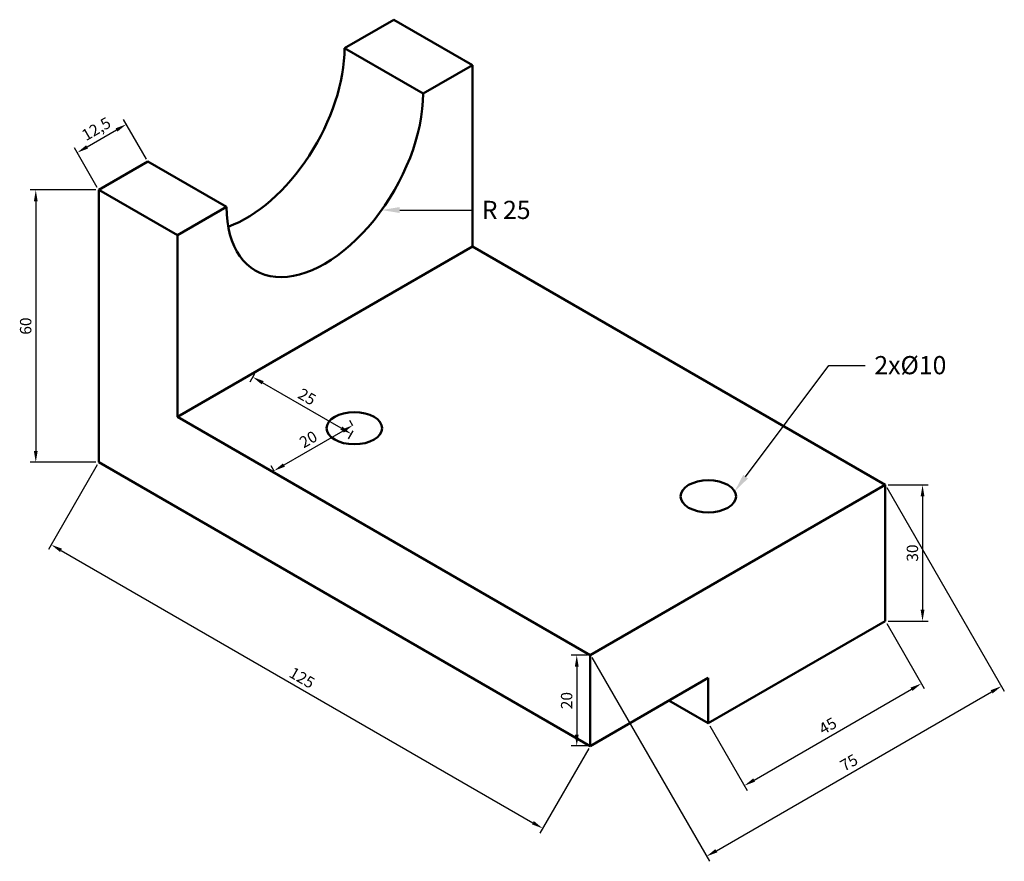
# Model space of a CAD drawing. Units: millimetres. Extents: x 163 to 380, y 64 to 249.
import ezdxf
from ezdxf import colors
from ezdxf.entities.mleader import LeaderData, LeaderLine
from ezdxf.math import Vec2, Vec3

# ---------------------------------------------------------------- set-up
doc = ezdxf.new("R2010")
doc.units = ezdxf.units.MM
for name, color, linetype, lineweight in [('M-DIMS', 2, 'Continuous', 25), ('M-OUTL', 7, 'Continuous', 50), ('M-TEXT', 3, 'Continuous', 25)]:
    doc.layers.add(name, color=color, linetype=linetype, lineweight=lineweight)
doc.styles.get("Standard").update_dxf_attribs({"font": 'arial.ttf'})
doc.dimstyles.new('ISO-25', dxfattribs={"dimtxt": 2.5, "dimasz": 2.5, "dimexe": 1.25, "dimexo": 0.625, "dimtad": 1, "dimtxsty": 'Standard', "dimcen": 2.5, "dimadec": 0, "dimazin": 0, "dimtfac": 1, "dimtmove": 0, "dimatfit": 3, "dimfxl": 1, "dimarcsym": 0})

# ---------------------------------------------------------------- blocks, each defined once
blk = doc.blocks.new('*D1')
at = {"layer": 'Defpoints', "color": 0, "transparency": 16777216}
for p in [(180.55, 211.41), (166.68, 151.41), (180.55, 151.41)]:
    blk.add_point(p, dxfattribs=at)
at = {"layer": 'M-DIMS', "color": 0, "lineweight": -2, "transparency": 16777216}
for p, q in [((179.92, 211.41), (165.43, 211.41)), ((166.68, 208.91), (166.68, 153.91)), ((179.92, 151.41), (165.43, 151.41))]:
    blk.add_line(p, q, dxfattribs=at)
at = {"layer": 'M-DIMS', "color": 0, "transparency": 16777216}
for points in [[(166.27, 208.91), (167.1, 208.91), (166.68, 211.41)], [(166.27, 153.91), (167.1, 153.91), (166.68, 151.41)]]:
    blk.add_solid(points, dxfattribs=at)
at = {"layer": 'M-DIMS', "color": 0, "transparency": 16777216, "insert": (164.78, 181.41), "char_height": 2.5, "attachment_point": 5, "rotation": 90}
blk.add_mtext('60', dxfattribs=at)
blk = doc.blocks.new('*D2')
at = {"layer": 'Defpoints', "color": 0, "transparency": 16777216}
for p in [(180.55, 151.41), (288.8, 88.91), (278.32, 70.76)]:
    blk.add_point(p, dxfattribs=at)
at = {"layer": 'M-DIMS', "color": 0, "lineweight": -2, "transparency": 16777216}
for p, q in [((180.23, 150.87), (169.45, 132.18)), ((172.24, 132.01), (276.16, 72.01)), ((288.49, 88.37), (277.7, 69.68))]:
    blk.add_line(p, q, dxfattribs=at)
at = {"layer": 'M-DIMS', "color": 0, "transparency": 16777216}
for points in [[(172.45, 132.37), (172.03, 131.65), (170.07, 133.26)], [(276.37, 72.37), (275.95, 71.65), (278.32, 70.76)]]:
    blk.add_solid(points, dxfattribs=at)
at = {"layer": 'M-DIMS', "color": 0, "transparency": 16777216, "insert": (225.15, 103.66), "char_height": 2.5, "attachment_point": 5, "rotation": 330}
blk.add_mtext('125', dxfattribs=at)
blk = doc.blocks.new('*D3')
at = {"layer": 'Defpoints', "color": 0, "transparency": 16777216}
for p in [(353.75, 116.41), (361.69, 102.66), (314.78, 93.91)]:
    blk.add_point(p, dxfattribs=at)
at = {"layer": 'M-DIMS', "color": 0, "lineweight": -2, "transparency": 16777216}
for p, q in [((354.06, 115.87), (362.31, 101.58)), ((324.88, 81.41), (359.52, 101.41)), ((315.09, 93.37), (323.34, 79.08))]:
    blk.add_line(p, q, dxfattribs=at)
at = {"layer": 'M-DIMS', "color": 0, "transparency": 16777216}
for points in [[(359.31, 101.78), (359.73, 101.05), (361.69, 102.66)], [(324.67, 81.78), (325.09, 81.05), (322.72, 80.16)]]:
    blk.add_solid(points, dxfattribs=at)
at = {"layer": 'M-DIMS', "color": 0, "transparency": 16777216, "insert": (341.25, 93.06), "char_height": 2.5, "attachment_point": 5, "rotation": 30}
blk.add_mtext('45', dxfattribs=at)
blk = doc.blocks.new('*D4')
at = {"layer": 'Defpoints', "color": 0, "transparency": 16777216}
for p in [(288.8, 108.91), (285.81, 88.91), (288.8, 88.91)]:
    blk.add_point(p, dxfattribs=at)
at = {"layer": 'M-DIMS', "color": 0, "lineweight": -2, "transparency": 16777216}
for p, q in [((288.18, 108.91), (284.56, 108.91)), ((285.81, 106.41), (285.81, 91.41)), ((288.18, 88.91), (284.56, 88.91))]:
    blk.add_line(p, q, dxfattribs=at)
at = {"layer": 'M-DIMS', "color": 0, "transparency": 16777216}
for points in [[(285.4, 106.41), (286.23, 106.41), (285.81, 108.91)], [(285.4, 91.41), (286.23, 91.41), (285.81, 88.91)]]:
    blk.add_solid(points, dxfattribs=at)
at = {"layer": 'M-DIMS', "color": 0, "transparency": 16777216, "insert": (283.91, 98.91), "char_height": 2.5, "attachment_point": 5, "rotation": 90}
blk.add_mtext('20', dxfattribs=at)
blk = doc.blocks.new('*D5')
at = {"layer": 'Defpoints', "color": 0, "transparency": 16777216}
for p in [(236.84, 158.91), (219.15, 149.54), (219.52, 148.91)]:
    blk.add_point(p, dxfattribs=at)
at = {"layer": 'M-DIMS', "color": 0, "lineweight": -2, "transparency": 16777216}
for p, q in [((236.53, 159.45), (235.85, 160.62)), ((234.31, 158.29), (221.32, 150.79)), ((219.21, 149.45), (218.53, 150.62))]:
    blk.add_line(p, q, dxfattribs=at)
at = {"layer": 'M-DIMS', "color": 0, "transparency": 16777216}
for points in [[(234.1, 158.65), (234.52, 157.93), (236.47, 159.54)], [(221.11, 151.15), (221.53, 150.43), (219.15, 149.54)]]:
    blk.add_solid(points, dxfattribs=at)
at = {"layer": 'M-DIMS', "color": 0, "transparency": 16777216, "insert": (226.86, 156.19), "char_height": 2.5, "attachment_point": 5, "rotation": 30}
blk.add_mtext('20', dxfattribs=at)
blk = doc.blocks.new('*D6')
at = {"layer": 'Defpoints', "color": 0, "transparency": 16777216}
for p in [(215.19, 171.41), (214.48, 170.18), (236.84, 158.91)]:
    blk.add_point(p, dxfattribs=at)
at = {"layer": 'M-DIMS', "color": 0, "lineweight": -2, "transparency": 16777216}
for p, q in [((214.88, 170.87), (213.85, 169.09)), ((233.96, 158.93), (216.64, 168.93)), ((236.53, 158.37), (235.5, 156.59))]:
    blk.add_line(p, q, dxfattribs=at)
at = {"layer": 'M-DIMS', "color": 0, "transparency": 16777216}
for points in [[(216.85, 169.29), (216.43, 168.56), (214.48, 170.18)], [(234.17, 159.29), (233.75, 158.56), (236.13, 157.68)]]:
    blk.add_solid(points, dxfattribs=at)
at = {"layer": 'M-DIMS', "color": 0, "transparency": 16777216, "insert": (226.25, 165.57), "char_height": 2.5, "attachment_point": 5, "rotation": 330}
blk.add_mtext('25', dxfattribs=at)
blk = doc.blocks.new('*D7')
at = {"layer": 'Defpoints', "color": 0, "transparency": 16777216}
for p in [(353.75, 146.41), (288.8, 108.91), (379.34, 102.09)]:
    blk.add_point(p, dxfattribs=at)
at = {"layer": 'M-DIMS', "color": 0, "lineweight": -2, "transparency": 16777216}
for p, q in [((354.06, 145.87), (379.96, 101.01)), ((289.11, 108.37), (315.01, 63.51)), ((316.55, 65.84), (377.17, 100.84))]:
    blk.add_line(p, q, dxfattribs=at)
at = {"layer": 'M-DIMS', "color": 0, "transparency": 16777216}
for points in [[(376.97, 101.2), (377.38, 100.48), (379.34, 102.09)], [(316.34, 66.2), (316.76, 65.48), (314.39, 64.59)]]:
    blk.add_solid(points, dxfattribs=at)
at = {"layer": 'M-DIMS', "color": 0, "transparency": 16777216, "insert": (345.91, 84.98), "char_height": 2.5, "attachment_point": 5, "rotation": 30}
blk.add_mtext('75', dxfattribs=at)
blk = doc.blocks.new('*D8')
at = {"layer": 'Defpoints', "color": 0, "transparency": 16777216}
for p in [(353.75, 146.41), (353.75, 116.41), (361.96, 116.41)]:
    blk.add_point(p, dxfattribs=at)
at = {"layer": 'M-DIMS', "color": 0, "lineweight": -2, "transparency": 16777216}
for p, q in [((354.38, 146.41), (363.21, 146.41)), ((361.96, 143.91), (361.96, 118.91)), ((354.38, 116.41), (363.21, 116.41))]:
    blk.add_line(p, q, dxfattribs=at)
at = {"layer": 'M-DIMS', "color": 0, "transparency": 16777216}
for points in [[(361.54, 143.91), (362.37, 143.91), (361.96, 146.41)], [(361.54, 118.91), (362.37, 118.91), (361.96, 116.41)]]:
    blk.add_solid(points, dxfattribs=at)
at = {"layer": 'M-DIMS', "color": 0, "transparency": 16777216, "insert": (360.05, 131.41), "char_height": 2.5, "attachment_point": 5, "rotation": 90}
blk.add_mtext('30', dxfattribs=at)
blk = doc.blocks.new('*D9')
at = {"layer": 'Defpoints', "color": 0, "transparency": 16777216}
for p in [(186.63, 225.87), (191.37, 217.66), (180.55, 211.41)]:
    blk.add_point(p, dxfattribs=at)
at = {"layer": 'M-DIMS', "color": 0, "lineweight": -2, "transparency": 16777216}
for p, q in [((191.06, 218.2), (186.01, 226.95)), ((177.97, 220.87), (184.47, 224.62)), ((180.23, 211.95), (175.18, 220.7))]:
    blk.add_line(p, q, dxfattribs=at)
at = {"layer": 'M-DIMS', "color": 0, "transparency": 16777216}
for points in [[(184.26, 224.98), (184.68, 224.26), (186.63, 225.87)], [(177.76, 221.23), (178.18, 220.51), (175.81, 219.62)]]:
    blk.add_solid(points, dxfattribs=at)
at = {"layer": 'M-DIMS', "color": 0, "transparency": 16777216, "insert": (180.16, 224.58), "char_height": 2.5, "attachment_point": 5, "rotation": 30}
blk.add_mtext('12,5', dxfattribs=at)

msp = doc.modelspace()

# ---------------------------------------------------------------- linework, layer by layer
at = {"layer": 'M-OUTL'}
for p, q in [((245.499, 248.907), (234.674, 242.657)), ((262.819, 238.907), (245.499, 248.907)), ((234.674, 242.657), (251.994, 232.657)), ((251.994, 232.657), (262.819, 238.907)), ((262.819, 198.907), (262.819, 238.907)), ((191.372, 217.657), (180.547, 211.407)), ((191.372, 217.657), (208.693, 207.657)), ((180.547, 151.407), (180.547, 211.407)), ((180.547, 211.407), (197.867, 201.407)), ((197.867, 201.407), (208.693, 207.657)), ((197.867, 201.407), (197.867, 161.407)), ((197.867, 161.407), (262.819, 198.907)), ((353.752, 146.407), (262.819, 198.907)), ((197.867, 161.407), (288.8, 108.907)), ((180.547, 151.407), (288.8, 88.907)), ((288.8, 108.907), (353.752, 146.407)), ((353.752, 116.407), (353.752, 146.407)), ((314.781, 93.907), (353.752, 116.407)), ((288.8, 108.907), (288.8, 88.907)), ((288.8, 88.907), (314.781, 103.907)), ((314.781, 103.907), (314.781, 93.907)), ((314.781, 93.907), (306.121, 98.907))]:
    msp.add_line(p, q, dxfattribs=at)
for centre, start_param in [((213.023, 230.157), 6.8844495), ((230.343, 220.157), 5.4977871)]:
    msp.add_ellipse(centre, major_axis=(-15.309, -26.517), ratio=0.5773503, start_param=start_param, end_param=8.6393798, dxfattribs=at)
for centre in [(236.839, 158.907), (314.781, 143.907)]:
    msp.add_ellipse(centre, major_axis=(-6.124, 0), ratio=0.5773503, dxfattribs=at)

# ---------------------------------------------------------------- dimensions: what is measured, and where the dimension line sits
at = {"layer": 'M-DIMS'}
for p1, p2, distance, picture, middle in [((180.547, 211.407), (191.372, 217.657), 9.479, '*D9', (180.156, 224.584)), ((236.839, 158.907), (215.188, 171.407), 1.423, '*D6', (226.253, 165.572)), ((236.839, 158.907), (219.518, 148.907), -0.729, '*D5', (226.863, 156.185)), ((180.547, 151.407), (288.8, 88.907), -20.951, '*D2', (225.149, 103.66)), ((288.8, 108.907), (353.752, 146.407), -51.174, '*D7', (345.915, 84.982)), ((314.781, 93.907), (353.752, 116.407), -15.869, '*D3', (341.253, 93.057))]:
    dim = msp.add_aligned_dim(p1=p1, p2=p2, distance=distance, dimstyle='ISO-25', override={"dimclrd": 0, "dimclre": 0, "dimclrt": 0}, dxfattribs=at)
    dim.commit()
    dim.dimension.update_dxf_attribs({"geometry": picture, "text_midpoint": middle})
for base, p1, p2, picture, middle in [((166.683, 151.407), (180.547, 211.407), (180.547, 151.407), '*D1', (164.782, 181.407)), ((361.956, 116.407), (353.752, 146.407), (353.752, 116.407), '*D8', (360.054, 131.407)), ((285.814, 88.907), (288.8, 108.907), (288.8, 88.907), '*D4', (283.912, 98.907))]:
    dim = msp.add_linear_dim(base=base, p1=p1, p2=p2, angle=90, dimstyle='ISO-25', override={"dimclrd": 0, "dimclre": 0, "dimclrt": 0}, dxfattribs=at)
    dim.commit()
    dim.dimension.update_dxf_attribs({"geometry": picture, "text_midpoint": middle})

# ---------------------------------------------------------------- leaders
at = {"layer": 'M-TEXT'}
ml = msp.add_multileader_mtext('Standard', dxfattribs=at)
ml.set_content('R 25', color=256)
ml.set_leader_properties()
ml.build(insert=Vec2(0, 0))
ctx = ml.context
ctx.base_point, ctx.plane_origin = Vec3(262.892, 206.973), Vec3(242.852, 206.973)
notes = []
notes.append((ctx, [(0, (1, 1, 0), (254.892, 206.973), (1, 0), 8, [(0, [(242.852, 206.973)], 0, [])])]))
ctx.mtext.insert, ctx.mtext.flow_direction = Vec3(264.892, 209.007), 5
ml = msp.add_multileader_mtext('Standard', dxfattribs=at)
ml.set_content('2x%%C10', color=256)
ml.set_leader_properties()
ml.build(insert=Vec2(0, 0))
ctx = ml.context
ctx.base_point, ctx.plane_origin = Vec3(349.353, 172.726), Vec3(320.589, 145.028)
notes.append((ctx, [(0, (1, 1, 0), (341.353, 172.726), (1, 0), 8, [(0, [(320.589, 145.028)], 0, [])])]))
ctx.mtext.insert, ctx.mtext.flow_direction = Vec3(351.353, 174.806), 5
for ctx, leaders in notes:
    for number, flags, end, landing, length, lines in leaders:
        leader = LeaderData()
        leader.index, (leader.has_last_leader_line, leader.has_dogleg_vector, leader.attachment_direction) = number, flags
        leader.last_leader_point, leader.dogleg_vector, leader.dogleg_length = Vec3(end), Vec3(landing), length
        for number, points, colour, breaks in lines:
            line = LeaderLine()
            line.index, line.vertices, line.color, line.breaks = number, Vec3.list(points), colors.encode_raw_color(colour), breaks
            leader.lines.append(line)
        ctx.leaders.append(leader)

doc.saveas('drawing.dxf')
